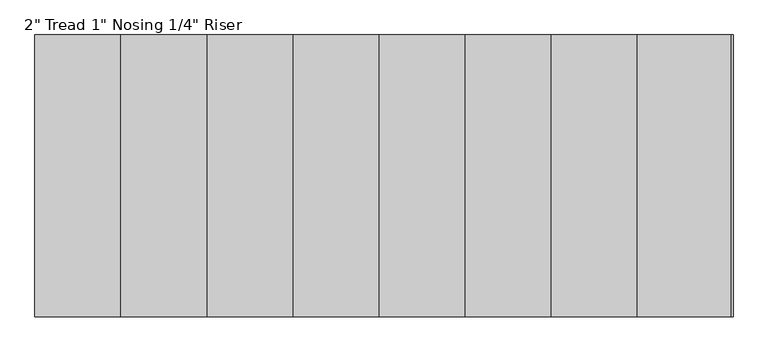
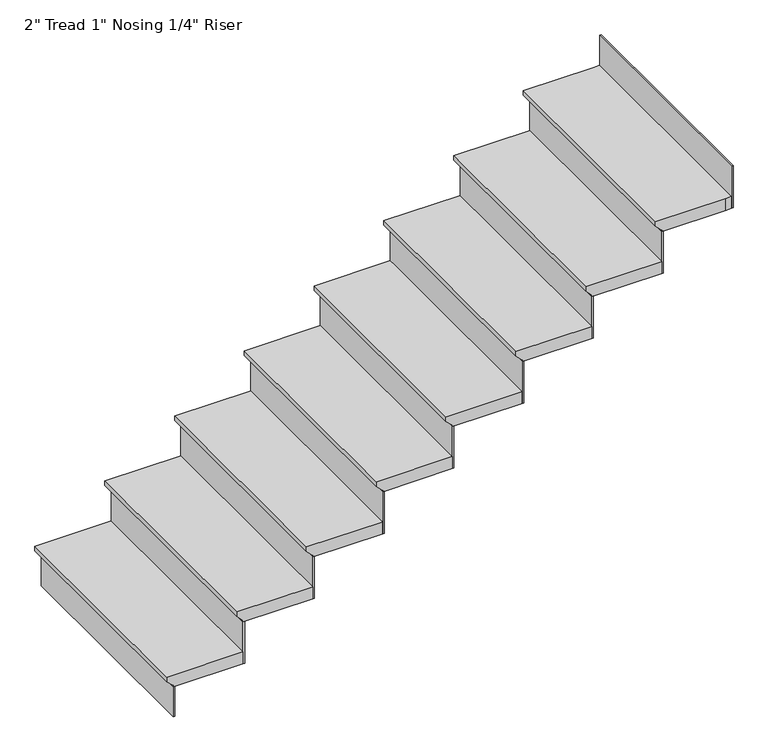
"""IFC4 building model written with IfcOpenShell, lengths in millimetres: stair flight geometry."""

from ifc_helpers import new_model, si_unit, origin, place, context, project, spatial, faceted_brep, source, transform, mapped, element, save


def stair_flight_fd6a9547(model_context):
    return source(origin(), model_context, "Body", "Brep", [
        faceted_brep([(6584.2175025, 6928.6147181, 768.35), (6584.2175025, 6928.6147181, 787.4), (6584.2175025, 7843.0147181, 787.4), (6584.2175025, 7843.0147181, 768.35), (6609.6175025, 6928.6147181, 742.95), (6609.6175025, 7843.0147181, 742.95), (6889.0175025, 6928.6147181, 787.4), (6889.0175025, 7843.0147181, 787.4), (6609.6175025, 7843.0147181, 736.6), (6889.0175025, 7843.0147181, 736.6), (6889.0175025, 6928.6147181, 736.6), (6609.6175025, 6928.6147181, 736.6)], [[[0, 1, 2, 3]], [[4, 0, 3, 5]], [[2, 1, 6, 7]], [[8, 9, 10, 11]], [[2, 7, 9, 8, 5, 3]], [[8, 11, 4, 5]], [[6, 1, 0, 4, 11, 10]], [[7, 6, 10, 9]]]),
        faceted_brep([(6609.6175025, 6928.6147181, 736.6), (6609.6175025, 6928.6147181, 609.6), (6615.9675025, 6928.6147181, 609.6), (6615.9675025, 6928.6147181, 736.6), (6609.6175025, 7843.0147181, 736.6), (6615.9675025, 7843.0147181, 736.6), (6615.9675025, 7843.0147181, 609.6), (6609.6175025, 7843.0147181, 609.6)], [[[0, 1, 2, 3]], [[4, 5, 6, 7]], [[1, 0, 4, 7]], [[2, 1, 7, 6]], [[3, 2, 6, 5]], [[0, 3, 5, 4]]]),
        faceted_brep([(6889.0175025, 6928.6147181, 914.4), (6889.0175025, 6928.6147181, 736.6), (6895.3675025, 6928.6147181, 736.6), (6895.3675025, 6928.6147181, 914.4), (6889.0175025, 7843.0147181, 914.4), (6895.3675025, 7843.0147181, 914.4), (6895.3675025, 7843.0147181, 736.6), (6889.0175025, 7843.0147181, 736.6)], [[[0, 1, 2, 3]], [[4, 5, 6, 7]], [[1, 0, 4, 7]], [[2, 1, 7, 6]], [[3, 2, 6, 5]], [[0, 3, 5, 4]]]),
        faceted_brep([(6863.6175025, 7843.0147181, 965.2), (6863.6175025, 6928.6147181, 965.2), (7168.4175025, 6928.6147181, 965.2), (7168.4175025, 7843.0147181, 965.2), (6889.0175025, 7843.0147181, 914.4), (7168.4175025, 7843.0147181, 914.4), (7168.4175025, 6928.6147181, 914.4), (6889.0175025, 6928.6147181, 914.4), (6889.0175025, 7843.0147181, 920.75), (6863.6175025, 7843.0147181, 946.15), (6889.0175025, 6928.6147181, 920.75), (6863.6175025, 6928.6147181, 946.15)], [[[0, 1, 2, 3]], [[4, 5, 6, 7]], [[0, 3, 5, 4, 8, 9]], [[4, 7, 10, 8]], [[2, 1, 11, 10, 7, 6]], [[3, 2, 6, 5]], [[11, 1, 0, 9]], [[10, 11, 9, 8]]]),
        faceted_brep([(7168.4175025, 6928.6147181, 1092.2), (7168.4175025, 6928.6147181, 914.4), (7174.7675025, 6928.6147181, 914.4), (7174.7675025, 6928.6147181, 1092.2), (7168.4175025, 7843.0147181, 1092.2), (7174.7675025, 7843.0147181, 1092.2), (7174.7675025, 7843.0147181, 914.4), (7168.4175025, 7843.0147181, 914.4)], [[[0, 1, 2, 3]], [[4, 5, 6, 7]], [[1, 0, 4, 7]], [[2, 1, 7, 6]], [[3, 2, 6, 5]], [[0, 3, 5, 4]]]),
        faceted_brep([(7143.0175025, 7843.0147181, 1143.0), (7143.0175025, 6928.6147181, 1143.0), (7447.8175025, 6928.6147181, 1143.0), (7447.8175025, 7843.0147181, 1143.0), (7168.4175025, 7843.0147181, 1092.2), (7447.8175025, 7843.0147181, 1092.2), (7447.8175025, 6928.6147181, 1092.2), (7168.4175025, 6928.6147181, 1092.2), (7168.4175025, 7843.0147181, 1098.55), (7143.0175025, 7843.0147181, 1123.95), (7168.4175025, 6928.6147181, 1098.55), (7143.0175025, 6928.6147181, 1123.95)], [[[0, 1, 2, 3]], [[4, 5, 6, 7]], [[0, 3, 5, 4, 8, 9]], [[4, 7, 10, 8]], [[2, 1, 11, 10, 7, 6]], [[3, 2, 6, 5]], [[11, 1, 0, 9]], [[10, 11, 9, 8]]]),
        faceted_brep([(7447.8175025, 6928.6147181, 1270.0), (7447.8175025, 6928.6147181, 1092.2), (7454.1675025, 6928.6147181, 1092.2), (7454.1675025, 6928.6147181, 1270.0), (7447.8175025, 7843.0147181, 1270.0), (7454.1675025, 7843.0147181, 1270.0), (7454.1675025, 7843.0147181, 1092.2), (7447.8175025, 7843.0147181, 1092.2)], [[[0, 1, 2, 3]], [[4, 5, 6, 7]], [[1, 0, 4, 7]], [[2, 1, 7, 6]], [[3, 2, 6, 5]], [[0, 3, 5, 4]]]),
        faceted_brep([(7422.4175025, 7843.0147181, 1320.8), (7422.4175025, 6928.6147181, 1320.8), (7727.2175025, 6928.6147181, 1320.8), (7727.2175025, 7843.0147181, 1320.8), (7447.8175025, 7843.0147181, 1270.0), (7727.2175025, 7843.0147181, 1270.0), (7727.2175025, 6928.6147181, 1270.0), (7447.8175025, 6928.6147181, 1270.0), (7447.8175025, 7843.0147181, 1276.35), (7422.4175025, 7843.0147181, 1301.75), (7447.8175025, 6928.6147181, 1276.35), (7422.4175025, 6928.6147181, 1301.75)], [[[0, 1, 2, 3]], [[4, 5, 6, 7]], [[0, 3, 5, 4, 8, 9]], [[4, 7, 10, 8]], [[2, 1, 11, 10, 7, 6]], [[3, 2, 6, 5]], [[11, 1, 0, 9]], [[10, 11, 9, 8]]]),
        faceted_brep([(7727.2175025, 6928.6147181, 1447.8), (7727.2175025, 6928.6147181, 1270.0), (7733.5675025, 6928.6147181, 1270.0), (7733.5675025, 6928.6147181, 1447.8), (7727.2175025, 7843.0147181, 1447.8), (7733.5675025, 7843.0147181, 1447.8), (7733.5675025, 7843.0147181, 1270.0), (7727.2175025, 7843.0147181, 1270.0)], [[[0, 1, 2, 3]], [[4, 5, 6, 7]], [[1, 0, 4, 7]], [[2, 1, 7, 6]], [[3, 2, 6, 5]], [[0, 3, 5, 4]]]),
        faceted_brep([(7701.8175025, 7843.0147181, 1498.6), (7701.8175025, 6928.6147181, 1498.6), (8006.6175025, 6928.6147181, 1498.6), (8006.6175025, 7843.0147181, 1498.6), (7727.2175025, 7843.0147181, 1447.8), (8006.6175025, 7843.0147181, 1447.8), (8006.6175025, 6928.6147181, 1447.8), (7727.2175025, 6928.6147181, 1447.8), (7727.2175025, 7843.0147181, 1454.15), (7701.8175025, 7843.0147181, 1479.55), (7727.2175025, 6928.6147181, 1454.15), (7701.8175025, 6928.6147181, 1479.55)], [[[0, 1, 2, 3]], [[4, 5, 6, 7]], [[0, 3, 5, 4, 8, 9]], [[4, 7, 10, 8]], [[2, 1, 11, 10, 7, 6]], [[3, 2, 6, 5]], [[11, 1, 0, 9]], [[10, 11, 9, 8]]]),
        faceted_brep([(8006.6175025, 6928.6147181, 1625.6), (8006.6175025, 6928.6147181, 1447.8), (8012.9675025, 6928.6147181, 1447.8), (8012.9675025, 6928.6147181, 1625.6), (8006.6175025, 7843.0147181, 1625.6), (8012.9675025, 7843.0147181, 1625.6), (8012.9675025, 7843.0147181, 1447.8), (8006.6175025, 7843.0147181, 1447.8)], [[[0, 1, 2, 3]], [[4, 5, 6, 7]], [[1, 0, 4, 7]], [[2, 1, 7, 6]], [[3, 2, 6, 5]], [[0, 3, 5, 4]]]),
        faceted_brep([(7981.2175025, 7843.0147181, 1676.4), (7981.2175025, 6928.6147181, 1676.4), (8286.0175025, 6928.6147181, 1676.4), (8286.0175025, 7843.0147181, 1676.4), (8006.6175025, 7843.0147181, 1625.6), (8286.0175025, 7843.0147181, 1625.6), (8286.0175025, 6928.6147181, 1625.6), (8006.6175025, 6928.6147181, 1625.6), (8006.6175025, 7843.0147181, 1631.95), (7981.2175025, 7843.0147181, 1657.35), (8006.6175025, 6928.6147181, 1631.95), (7981.2175025, 6928.6147181, 1657.35)], [[[0, 1, 2, 3]], [[4, 5, 6, 7]], [[0, 3, 5, 4, 8, 9]], [[4, 7, 10, 8]], [[2, 1, 11, 10, 7, 6]], [[3, 2, 6, 5]], [[11, 1, 0, 9]], [[10, 11, 9, 8]]]),
        faceted_brep([(8286.0175025, 6928.6147181, 1803.4), (8286.0175025, 6928.6147181, 1625.6), (8292.3675025, 6928.6147181, 1625.6), (8292.3675025, 6928.6147181, 1803.4), (8286.0175025, 7843.0147181, 1803.4), (8292.3675025, 7843.0147181, 1803.4), (8292.3675025, 7843.0147181, 1625.6), (8286.0175025, 7843.0147181, 1625.6)], [[[0, 1, 2, 3]], [[4, 5, 6, 7]], [[1, 0, 4, 7]], [[2, 1, 7, 6]], [[3, 2, 6, 5]], [[0, 3, 5, 4]]]),
        faceted_brep([(8260.6175025, 7843.0147181, 1854.2), (8260.6175025, 6928.6147181, 1854.2), (8565.4175025, 6928.6147181, 1854.2), (8565.4175025, 7843.0147181, 1854.2), (8286.0175025, 7843.0147181, 1803.4), (8565.4175025, 7843.0147181, 1803.4), (8565.4175025, 6928.6147181, 1803.4), (8286.0175025, 6928.6147181, 1803.4), (8286.0175025, 7843.0147181, 1809.75), (8260.6175025, 7843.0147181, 1835.15), (8286.0175025, 6928.6147181, 1809.75), (8260.6175025, 6928.6147181, 1835.15)], [[[0, 1, 2, 3]], [[4, 5, 6, 7]], [[0, 3, 5, 4, 8, 9]], [[4, 7, 10, 8]], [[2, 1, 11, 10, 7, 6]], [[3, 2, 6, 5]], [[11, 1, 0, 9]], [[10, 11, 9, 8]]]),
        faceted_brep([(8844.8175025, 6928.6147181, 2159.0), (8844.8175025, 6928.6147181, 1981.2), (8851.1675025, 6928.6147181, 1981.2), (8851.1675025, 6928.6147181, 2159.0), (8844.8175025, 7843.0147181, 2159.0), (8851.1675025, 7843.0147181, 2159.0), (8851.1675025, 7843.0147181, 1981.2), (8844.8175025, 7843.0147181, 1981.2)], [[[0, 1, 2, 3]], [[4, 5, 6, 7]], [[1, 0, 4, 7]], [[2, 1, 7, 6]], [[3, 2, 6, 5]], [[0, 3, 5, 4]]]),
        faceted_brep([(8565.4175025, 6928.6147181, 1981.2), (8565.4175025, 6928.6147181, 1803.4), (8571.7675025, 6928.6147181, 1803.4), (8571.7675025, 6928.6147181, 1981.2), (8565.4175025, 7843.0147181, 1981.2), (8571.7675025, 7843.0147181, 1981.2), (8571.7675025, 7843.0147181, 1803.4), (8565.4175025, 7843.0147181, 1803.4)], [[[0, 1, 2, 3]], [[4, 5, 6, 7]], [[1, 0, 4, 7]], [[2, 1, 7, 6]], [[3, 2, 6, 5]], [[0, 3, 5, 4]]]),
        faceted_brep([(8844.8175025, 7843.0147181, 2032.0), (8819.4175025, 7843.0147181, 2032.0), (8540.0175025, 7843.0147181, 2032.0), (8540.0175025, 6928.6147181, 2032.0), (8819.4175025, 6928.6147181, 2032.0), (8844.8175025, 6928.6147181, 2032.0), (8819.4175025, 7843.0147181, 1981.2), (8844.8175025, 7843.0147181, 1981.2), (8844.8175025, 6928.6147181, 1981.2), (8819.4175025, 6928.6147181, 1981.2), (8565.4175025, 6928.6147181, 1981.2), (8565.4175025, 7843.0147181, 1981.2), (8565.4175025, 7843.0147181, 1987.55), (8540.0175025, 7843.0147181, 2012.95), (8565.4175025, 6928.6147181, 1987.55), (8540.0175025, 6928.6147181, 2012.95)], [[[0, 1, 2, 3, 4, 5]], [[6, 7, 8, 9, 10, 11]], [[1, 0, 7, 6]], [[2, 1, 6, 11, 12, 13]], [[11, 10, 14, 12]], [[4, 3, 15, 14, 10, 9]], [[5, 4, 9, 8]], [[0, 5, 8, 7]], [[15, 3, 2, 13]], [[14, 15, 13, 12]]]),
    ])


if __name__ == "__main__":
    model = new_model("IFC4")
    model_context = context("Model", 3, world=origin())
    ifc_project = project(units=[si_unit("LENGTHUNIT", "METRE", prefix="MILLI")], contexts=[model_context])
    site = spatial("IfcSite", under=ifc_project)
    building = spatial("IfcBuilding", under=site)
    placement = place(None, origin())
    stair_flight_shape = stair_flight_fd6a9547(model_context)
    element("IfcStairFlight", 1, ObjectType="2\" Tread 1\" Nosing 1/4\" Riser", at=placement, inside=building, context=model_context, shape_type="MappedRepresentation", body=[
        mapped(stair_flight_shape, transform((0.0, 0.0, 0.0), x_axis=(1.0, 0.0, 0.0), y_axis=(0.0, 1.0, 0.0), z_axis=(0.0, 0.0, 1.0))),
    ])
    save(model, "model.ifc")
